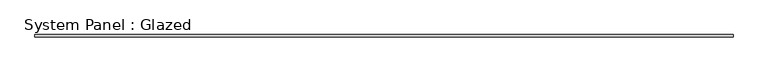
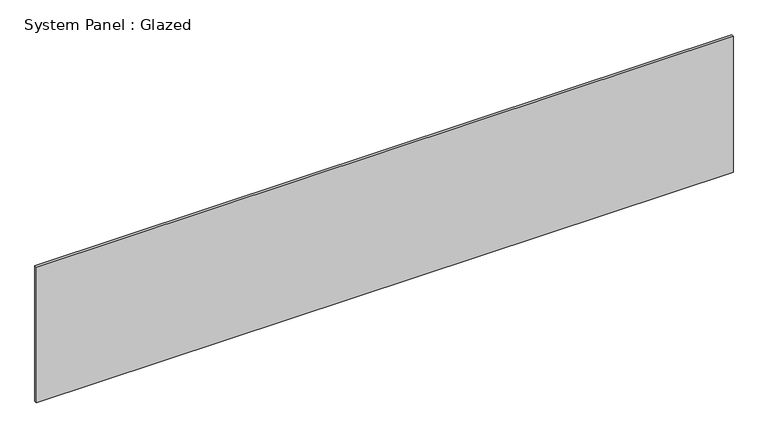
"""IFC4 building model written with IfcOpenShell, lengths in millimetres: plate geometry, System Panel : Glazed."""

from ifc_helpers import new_model, si_unit, origin, origin_with_axes, place, context, project, spatial, polyline, outline, extrude, source, transform, mapped, element, save


def system_panel_glazed_5985f842(model_context):
    return source(origin(), model_context, "Body", "SweptSolid", [
        extrude(outline(polyline([(3483.3971854, 19.05), (-3483.3971854, 19.05), (-3483.3971854, 44.45), (3483.3971854, 44.45), (3483.3971854, 19.05)])), origin_with_axes(), (0.0, 0.0, 1.0), 1435.862181),
    ])


if __name__ == "__main__":
    model = new_model("IFC4")
    model_context = context("Model", 3, world=origin())
    ifc_project = project(units=[si_unit("LENGTHUNIT", "METRE", prefix="MILLI")], contexts=[model_context])
    site = spatial("IfcSite", under=ifc_project)
    building = spatial("IfcBuilding", under=site)
    placement = place(None, origin())
    system_panel_glazed_shape = system_panel_glazed_5985f842(model_context)
    element("IfcPlate", 1, ObjectType="System Panel : Glazed", at=placement, inside=building, context=model_context, shape_type="MappedRepresentation", body=[
        mapped(system_panel_glazed_shape, transform((0.0, 0.0, 0.0), x_axis=(1.0, 0.0, 0.0), y_axis=(0.0, 1.0, 0.0), z_axis=(0.0, 0.0, 1.0))),
    ])
    save(model, "model.ifc")

# Revit data of these elements
# Type "System Panel : Glazed"
#   Construction Type Id = "GSP4R"
#   Analytic Construction = "1/8 in Pilkington single glazing"
#   Visual Light Transmittance = 0.9
#   Solar Heat Gain Coefficient = 0.86
#   Heat Transfer Coefficient (U) = 1.18115 BTU/(h·ft²·°F)
#   Define Thermal Properties by = 1
# Element 1 (IfcPlate, "System Panel : Glazed")
#   Materials on its faces: "Glass"
# Materials
#   "Glass": class "Glass", colour RGB 0 128 192, transparency 0.75, Description = "Soda Lime Glass", Cost = 0
